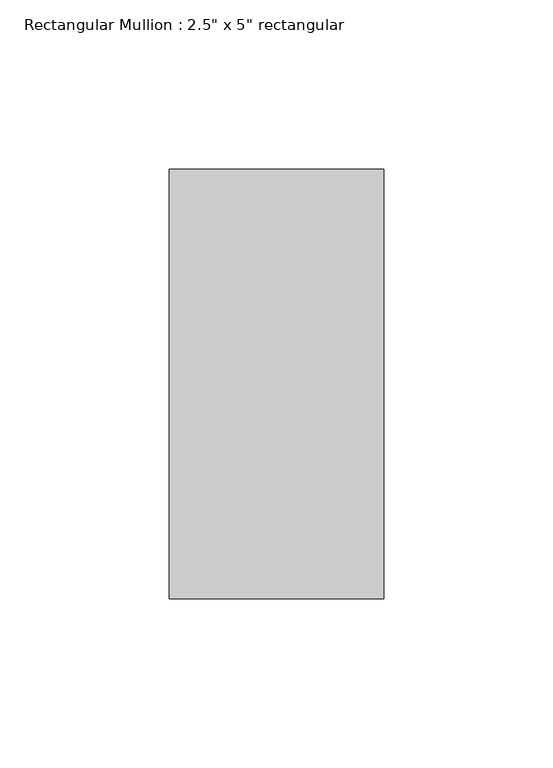
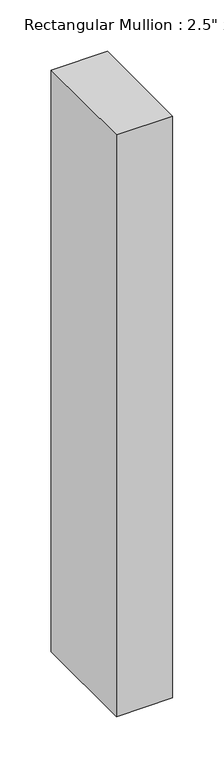
"""IFC4 building model written with IfcOpenShell, lengths in millimetres: member geometry."""

from ifc_helpers import new_model, si_unit, frame, origin, place, context, project, spatial, polyline, outline, extrude, source, transform, mapped, element, save


def member_675b1c02(model_context):
    return source(origin(), model_context, "Body", "SweptSolid", [
        extrude(outline(polyline([(0.0, 63.5), (0.0, -63.5), (-63.5, -63.5), (-63.5, 63.5), (0.0, 63.5)])), frame((0.0, 0.0, -691.8458312), z_axis=(0.0, 0.0, 1.0), x_axis=(1.0, 0.0, 0.0)), (0.0, 0.0, 1.0), 691.8458312),
    ])


if __name__ == "__main__":
    model = new_model("IFC4")
    model_context = context("Model", 3, world=origin())
    ifc_project = project(units=[si_unit("LENGTHUNIT", "METRE", prefix="MILLI")], contexts=[model_context])
    site = spatial("IfcSite", under=ifc_project)
    building = spatial("IfcBuilding", under=site)
    placement = place(None, origin())
    member_shape = member_675b1c02(model_context)
    element("IfcMember", 1, ObjectType="Rectangular Mullion : 2.5\" x 5\" rectangular", at=placement, inside=building, context=model_context, shape_type="MappedRepresentation", body=[
        mapped(member_shape, transform((0.0, 0.0, 0.0), x_axis=(1.0, 0.0, 0.0), y_axis=(0.0, 1.0, 0.0), z_axis=(0.0, 0.0, 1.0))),
    ])
    save(model, "model.ifc")

# Revit data of these elements
# Type "Rectangular Mullion : 2.5\" x 5\" rectangular"
#   built-in parameter 1007304 = 0.416667 (stored number, unit not read)
#   built-in parameter 1007301 = 0.104167 (stored number, unit not read)
#   built-in parameter 1007300 = 0.104167 (stored number, unit not read)
# Element 1 (IfcMember, "Rectangular Mullion : 2.5\" x 5\" rectangular")
#   Materials on its faces: "Aluminum"
# Materials
#   "Aluminum": class "Metal", colour RGB 247 247 247, transparency 0, Description = "Aluminum 6061", Cost = 0
